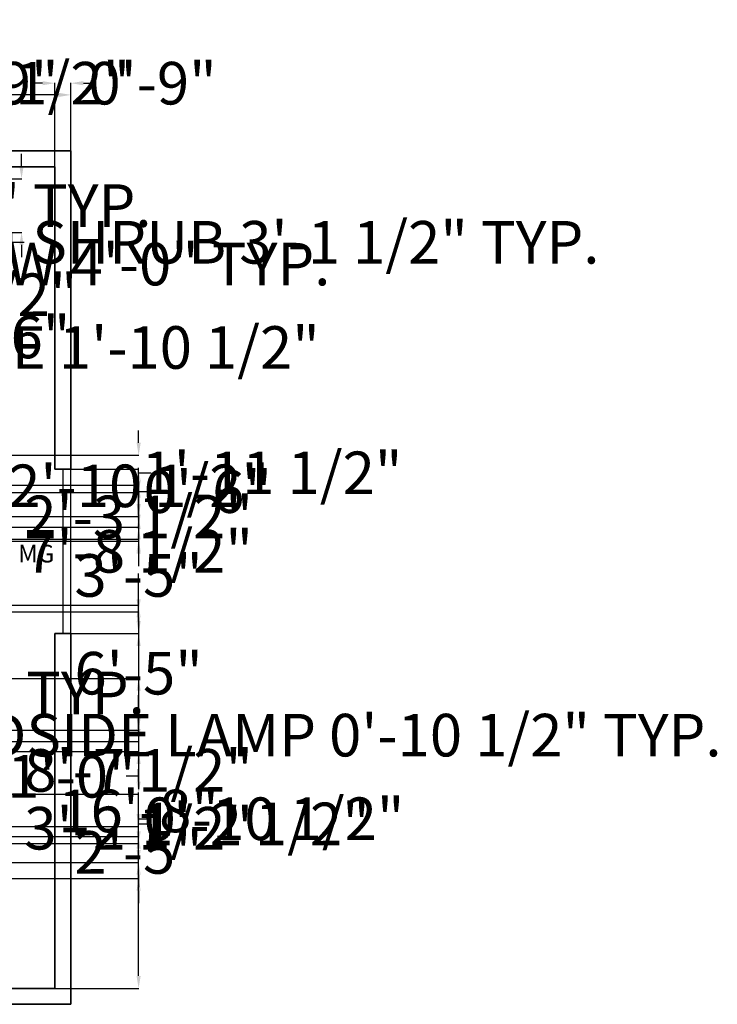
# Model space of a CAD drawing. Units: inches. Extents: x -166 to 1001, y 0 to 688.
# Tile 11 of 11: x 608 to 1001, y 74 to 629. Entities that reach past the tile are written whole.
import ezdxf

# ---------------------------------------------------------------- set-up
doc = ezdxf.new("R2010")
doc.units = ezdxf.units.IN
doc.header["$MEASUREMENT"] = 0
for name, color, linetype, lineweight in [('A-ANNO-DIMS', 1, 'Continuous', 18), ('A-ANNO-TEXT', 2, 'Continuous', 25), ('C-SITE-GATE', 250, 'Continuous', 25), ('C-SITE-WALL', 250, 'Continuous', 35)]:
    doc.layers.add(name, color=color, linetype=linetype, lineweight=lineweight)
doc.styles.get("Standard").update_dxf_attribs({"font": 'arial.ttf'})
doc.dimstyles.get("Standard").update_dxf_attribs({"dimtxt": 24, "dimasz": 7, "dimexe": 0.18, "dimexo": 0.0625, "dimgap": 0.09, "dimtad": 0, "dimtih": 1, "dimtoh": 1, "dimdec": 0, "dimzin": 0, "dimdsep": 46, "dimlunit": 3, "dimtxsty": 'Standard', "dimcen": 0.09, "dimadec": 0, "dimazin": 0, "dimtfac": 1, "dimtdec": 0, "dimtofl": 0, "dimtmove": 0, "dimatfit": 3, "dimfxl": 1, "dimtolj": 1, "dimtzin": 0, "dimarcsym": 0})

# ---------------------------------------------------------------- blocks, each defined once
blk = doc.blocks.new('*D10')
at = {"layer": 'A-ANNO-DIMS', "color": 0, "lineweight": -2, "transparency": 16777216}
for p, q in [((-82.62, 554.8), (-82.62, 586.48)), ((-75.62, 586.3), (256.61, 586.3)), ((629.88, 586.3), (297.65, 586.3)), ((636.88, 554.8), (636.88, 586.48))]:
    blk.add_line(p, q, dxfattribs=at)
at = {"layer": 'A-ANNO-DIMS', "color": 0, "transparency": 16777216}
for points in [[(-75.62, 587.47), (-75.62, 585.14), (-82.62, 586.3)], [(629.88, 587.47), (629.88, 585.14), (636.88, 586.3)]]:
    blk.add_solid(points, dxfattribs=at)
at = {"layer": 'Defpoints', "color": 0, "transparency": 16777216}
for p in [(636.88, 586.3), (-82.62, 554.74), (636.88, 554.74)]:
    blk.add_point(p, dxfattribs=at)
at = {"layer": 'A-ANNO-DIMS', "color": 0, "transparency": 16777216, "insert": (277.13, 586.3), "char_height": 24, "attachment_point": 5}
blk.add_mtext("\\A1;60'", dxfattribs=at)
blk = doc.blocks.new('*D15')
at = {"layer": 'A-ANNO-DIMS', "color": 0, "lineweight": -2, "transparency": 16777216}
for p, q in [((566.06, 508.76), (566.06, 503.04)), ((603.45, 508.76), (603.45, 503.04)), ((573.06, 503.22), (596.45, 503.22)), ((603.45, 503.22), (610.45, 503.22))]:
    blk.add_line(p, q, dxfattribs=at)
at = {"layer": 'A-ANNO-DIMS', "color": 0, "transparency": 16777216}
for points in [[(573.06, 504.38), (573.06, 502.05), (566.06, 503.22)], [(596.45, 504.38), (596.45, 502.05), (603.45, 503.22)]]:
    blk.add_solid(points, dxfattribs=at)
at = {"layer": 'Defpoints', "color": 0, "transparency": 16777216}
for p in [(566.06, 508.83), (603.45, 508.83), (603.45, 503.22)]:
    blk.add_point(p, dxfattribs=at)
at = {"layer": 'A-ANNO-DIMS', "color": 0, "transparency": 16777216, "insert": (774.93, 503.22), "char_height": 24, "attachment_point": 5}
blk.add_mtext('\\A1;SHRUB 3\'-1 1/2" TYP.', dxfattribs=at)
blk = doc.blocks.new('*D16')
at = {"layer": 'A-ANNO-DIMS', "color": 0, "lineweight": -2, "transparency": 16777216}
for p, q in [((609.06, 546), (609.06, 553)), ((603.51, 539), (609.24, 539)), ((603.51, 508.83), (609.24, 508.83)), ((609.06, 501.83), (609.06, 494.83))]:
    blk.add_line(p, q, dxfattribs=at)
at = {"layer": 'A-ANNO-DIMS', "color": 0, "transparency": 16777216}
for points in [[(607.89, 546), (610.23, 546), (609.06, 539)], [(607.89, 501.83), (610.23, 501.83), (609.06, 508.83)]]:
    blk.add_solid(points, dxfattribs=at)
at = {"layer": 'Defpoints', "color": 0, "transparency": 16777216}
for p in [(603.45, 539), (609.06, 539), (603.45, 508.83)]:
    blk.add_point(p, dxfattribs=at)
at = {"layer": 'A-ANNO-DIMS', "color": 0, "transparency": 16777216, "insert": (609.06, 523.91), "char_height": 24, "attachment_point": 5}
blk.add_mtext('\\A1;2\'-6" TYP.', dxfattribs=at)
blk = doc.blocks.new('*D17')
at = {"layer": 'A-ANNO-DIMS', "color": 0, "lineweight": -2, "transparency": 16777216}
for p, q in [((430.46, 483.8), (430.46, 491.12)), ((437.46, 490.94), (471.46, 490.94)), ((478.46, 483.8), (478.46, 491.12)), ((478.46, 490.94), (485.46, 490.94))]:
    blk.add_line(p, q, dxfattribs=at)
at = {"layer": 'A-ANNO-DIMS', "color": 0, "transparency": 16777216}
for points in [[(437.46, 492.11), (437.46, 489.77), (430.46, 490.94)], [(471.46, 492.11), (471.46, 489.77), (478.46, 490.94)]]:
    blk.add_solid(points, dxfattribs=at)
at = {"layer": 'Defpoints', "color": 0, "transparency": 16777216}
for p in [(478.46, 490.94), (430.46, 483.74), (478.46, 483.74)]:
    blk.add_point(p, dxfattribs=at)
at = {"layer": 'A-ANNO-DIMS', "color": 0, "transparency": 16777216, "insert": (637.4, 490.94), "char_height": 24, "attachment_point": 5}
blk.add_mtext('\\A1;WINDOW 4\'-0" TYP.', dxfattribs=at)
blk = doc.blocks.new('*D21')
at = {"layer": 'A-ANNO-DIMS', "color": 0, "lineweight": -2, "transparency": 16777216}
for p, q in [((506.04, 225.45), (499.04, 225.45)), ((513.04, 226.95), (513.04, 225.27)), ((523.44, 226.95), (523.44, 225.27)), ((530.44, 225.45), (537.44, 225.45))]:
    blk.add_line(p, q, dxfattribs=at)
at = {"layer": 'A-ANNO-DIMS', "color": 0, "transparency": 16777216}
for points in [[(506.04, 226.62), (506.04, 224.29), (513.04, 225.45)], [(530.44, 226.62), (530.44, 224.29), (523.44, 225.45)]]:
    blk.add_solid(points, dxfattribs=at)
at = {"layer": 'Defpoints', "color": 0, "transparency": 16777216}
for p in [(513.04, 227.01), (523.44, 227.01), (523.44, 225.45)]:
    blk.add_point(p, dxfattribs=at)
at = {"layer": 'A-ANNO-DIMS', "color": 0, "transparency": 16777216, "insert": (775.99, 225.45), "char_height": 24, "attachment_point": 5}
blk.add_mtext('\\A1;BEDSIDE LAMP 0\'-10 1/2" TYP.', dxfattribs=at)
blk = doc.blocks.new('*D22')
at = {"layer": 'A-ANNO-DIMS', "color": 0, "lineweight": -2, "transparency": 16777216}
for p, q in [((525, 242.21), (525, 249.21)), ((525, 249.21), (532, 249.21)), ((523.5, 235.21), (525.18, 235.21)), ((523.5, 227.01), (525.18, 227.01)), ((525, 220.01), (525, 213.01))]:
    blk.add_line(p, q, dxfattribs=at)
at = {"layer": 'A-ANNO-DIMS', "color": 0, "transparency": 16777216}
for points in [[(523.83, 242.21), (526.17, 242.21), (525, 235.21)], [(523.83, 220.01), (526.17, 220.01), (525, 227.01)]]:
    blk.add_solid(points, dxfattribs=at)
at = {"layer": 'Defpoints', "color": 0, "transparency": 16777216}
for p in [(523.44, 235.21), (525, 235.21), (523.44, 227.01)]:
    blk.add_point(p, dxfattribs=at)
at = {"layer": 'A-ANNO-DIMS', "color": 0, "transparency": 16777216, "insert": (605.24, 249.21), "char_height": 24, "attachment_point": 5}
blk.add_mtext('\\A1;0\'-8" TYP.', dxfattribs=at)
blk = doc.blocks.new('*D31')
at = {"layer": 'A-ANNO-DIMS', "color": 0, "lineweight": -2, "transparency": 16777216}
for p, q in [((484.56, 447.22), (484.56, 443.75)), ((506.92, 447.22), (506.92, 443.75)), ((491.56, 443.93), (499.92, 443.93)), ((506.92, 443.93), (513.92, 443.93))]:
    blk.add_line(p, q, dxfattribs=at)
at = {"layer": 'A-ANNO-DIMS', "color": 0, "transparency": 16777216}
for points in [[(491.56, 445.1), (491.56, 442.76), (484.56, 443.93)], [(499.92, 445.1), (499.92, 442.76), (506.92, 443.93)]]:
    blk.add_solid(points, dxfattribs=at)
at = {"layer": 'Defpoints', "color": 0, "transparency": 16777216}
for p in [(484.56, 447.28), (506.92, 447.28), (506.92, 443.93)]:
    blk.add_point(p, dxfattribs=at)
at = {"layer": 'A-ANNO-DIMS', "color": 0, "transparency": 16777216, "insert": (646.84, 443.93), "char_height": 24, "attachment_point": 5}
blk.add_mtext('\\A1;RANGE 1\'-10 1/2"', dxfattribs=at)
blk = doc.blocks.new('*D32')
at = {"layer": 'A-ANNO-DIMS', "color": 0, "lineweight": -2, "transparency": 16777216}
for p, q in [((510.27, 466.66), (510.27, 473.66)), ((510.27, 473.66), (517.27, 473.66)), ((506.98, 466.66), (510.45, 466.66)), ((510.27, 454.28), (510.27, 459.66)), ((506.98, 447.28), (510.45, 447.28))]:
    blk.add_line(p, q, dxfattribs=at)
at = {"layer": 'A-ANNO-DIMS', "color": 0, "transparency": 16777216}
for points in [[(509.1, 459.66), (511.44, 459.66), (510.27, 466.66)], [(509.1, 454.28), (511.44, 454.28), (510.27, 447.28)]]:
    blk.add_solid(points, dxfattribs=at)
at = {"layer": 'Defpoints', "color": 0, "transparency": 16777216}
for p in [(506.92, 466.66), (510.27, 466.66), (506.92, 447.28)]:
    blk.add_point(p, dxfattribs=at)
at = {"layer": 'A-ANNO-DIMS', "color": 0, "transparency": 16777216, "insert": (576.09, 473.66), "char_height": 24, "attachment_point": 5}
blk.add_mtext('\\A1;1\'-7 1/2"', dxfattribs=at)
blk = doc.blocks.new('*D33')
at = {"layer": 'A-ANNO-DIMS', "color": 0, "lineweight": -2, "transparency": 16777216}
for p, q in [((291.16, 438.23), (291.16, 450.03)), ((298.16, 449.85), (362.04, 449.85)), ((369.04, 438.23), (369.04, 450.03)), ((369.04, 449.85), (376.04, 449.85))]:
    blk.add_line(p, q, dxfattribs=at)
at = {"layer": 'A-ANNO-DIMS', "color": 0, "transparency": 16777216}
for points in [[(298.16, 451.02), (298.16, 448.68), (291.16, 449.85)], [(362.04, 451.02), (362.04, 448.68), (369.04, 449.85)]]:
    blk.add_solid(points, dxfattribs=at)
at = {"layer": 'Defpoints', "color": 0, "transparency": 16777216}
for p in [(369.04, 449.85), (291.16, 438.17), (369.04, 438.17)]:
    blk.add_point(p, dxfattribs=at)
at = {"layer": 'A-ANNO-DIMS', "color": 0, "transparency": 16777216, "insert": (508.03, 449.85), "char_height": 24, "attachment_point": 5}
blk.add_mtext('\\A1;DINING SET 6\'-6"', dxfattribs=at)
blk = doc.blocks.new('*D39')
at = {"layer": 'A-ANNO-DIMS', "color": 0, "lineweight": -2, "transparency": 16777216}
for p, q in [((627.94, 375.38), (675.21, 375.38)), ((675.03, 368.38), (675.03, 341.55)), ((675.03, 289.72), (675.03, 316.55)), ((627.94, 282.72), (675.21, 282.72))]:
    blk.add_line(p, q, dxfattribs=at)
at = {"layer": 'A-ANNO-DIMS', "color": 0, "transparency": 16777216}
for points in [[(673.87, 368.38), (676.2, 368.38), (675.03, 375.38)], [(673.87, 289.72), (676.2, 289.72), (675.03, 282.72)]]:
    blk.add_solid(points, dxfattribs=at)
at = {"layer": 'Defpoints', "color": 0, "transparency": 16777216}
for p in [(627.88, 375.38), (627.88, 282.72), (675.03, 282.72)]:
    blk.add_point(p, dxfattribs=at)
at = {"layer": 'A-ANNO-DIMS', "color": 0, "transparency": 16777216, "insert": (675.03, 329.05), "char_height": 24, "attachment_point": 5}
blk.add_mtext('\\A1;7\'-8 1/2"', dxfattribs=at)
blk = doc.blocks.new('*D40')
at = {"layer": 'A-ANNO-DIMS', "color": 0, "lineweight": -2, "transparency": 16777216}
for p, q in [((627.94, 282.72), (675.21, 282.72)), ((675.03, 275.72), (675.03, 195.07)), ((675.03, 89.74), (675.03, 170.38)), ((627.94, 82.74), (675.21, 82.74))]:
    blk.add_line(p, q, dxfattribs=at)
at = {"layer": 'A-ANNO-DIMS', "color": 0, "transparency": 16777216}
for points in [[(673.87, 275.72), (676.2, 275.72), (675.03, 282.72)], [(673.87, 89.74), (676.2, 89.74), (675.03, 82.74)]]:
    blk.add_solid(points, dxfattribs=at)
at = {"layer": 'Defpoints', "color": 0, "transparency": 16777216}
for p in [(627.88, 282.72), (675.03, 282.72), (627.88, 82.74)]:
    blk.add_point(p, dxfattribs=at)
at = {"layer": 'A-ANNO-DIMS', "color": 0, "transparency": 16777216, "insert": (675.03, 182.73), "char_height": 24, "attachment_point": 5}
blk.add_mtext('\\A1;16\'-8"', dxfattribs=at)
blk = doc.blocks.new('*D41')
at = {"layer": 'A-ANNO-DIMS', "color": 0, "lineweight": -2, "transparency": 16777216}
for p, q in [((620.88, 592.89), (613.88, 592.89)), ((627.88, 545.8), (627.88, 593.07)), ((636.88, 554.8), (636.88, 593.07)), ((643.88, 592.89), (650.88, 592.89))]:
    blk.add_line(p, q, dxfattribs=at)
at = {"layer": 'A-ANNO-DIMS', "color": 0, "transparency": 16777216}
for points in [[(620.88, 594.06), (620.88, 591.72), (627.88, 592.89)], [(643.88, 594.06), (643.88, 591.72), (636.88, 592.89)]]:
    blk.add_solid(points, dxfattribs=at)
at = {"layer": 'Defpoints', "color": 0, "transparency": 16777216}
for p in [(636.88, 592.89), (636.88, 554.74), (627.88, 545.74)]:
    blk.add_point(p, dxfattribs=at)
at = {"layer": 'A-ANNO-DIMS', "color": 0, "transparency": 16777216, "insert": (682.87, 592.89), "char_height": 24, "attachment_point": 5}
blk.add_mtext('\\A1;0\'-9"', dxfattribs=at)
blk = doc.blocks.new('*D47')
at = {"layer": 'A-ANNO-DIMS', "color": 0, "lineweight": -2, "transparency": 16777216}
for p, q in [((478.46, 483.8), (478.46, 593.07)), ((485.46, 592.89), (531.88, 592.89)), ((538.88, 483.8), (538.88, 593.07)), ((538.88, 592.89), (545.88, 592.89))]:
    blk.add_line(p, q, dxfattribs=at)
at = {"layer": 'A-ANNO-DIMS', "color": 0, "transparency": 16777216}
for points in [[(485.46, 594.06), (485.46, 591.72), (478.46, 592.89)], [(531.88, 594.06), (531.88, 591.72), (538.88, 592.89)]]:
    blk.add_solid(points, dxfattribs=at)
at = {"layer": 'Defpoints', "color": 0, "transparency": 16777216}
for p in [(538.88, 592.89), (478.46, 483.74), (538.88, 483.74)]:
    blk.add_point(p, dxfattribs=at)
at = {"layer": 'A-ANNO-DIMS', "color": 0, "transparency": 16777216, "insert": (605.83, 592.89), "char_height": 24, "attachment_point": 5}
blk.add_mtext('\\A1;5\'-0 1/2"', dxfattribs=at)
blk = doc.blocks.new('*D51')
at = {"layer": 'A-ANNO-DIMS', "color": 0, "lineweight": -2, "transparency": 16777216}
for p, q in [((675.03, 168.41), (675.03, 175.41)), ((675.03, 175.41), (682.03, 175.41)), ((24.44, 168.41), (675.21, 168.41)), ((675.03, 160.74), (675.03, 161.41)), ((24.44, 153.74), (675.21, 153.74))]:
    blk.add_line(p, q, dxfattribs=at)
at = {"layer": 'A-ANNO-DIMS', "color": 0, "transparency": 16777216}
for points in [[(673.87, 161.41), (676.2, 161.41), (675.03, 168.41)], [(673.87, 160.74), (676.2, 160.74), (675.03, 153.74)]]:
    blk.add_solid(points, dxfattribs=at)
at = {"layer": 'Defpoints', "color": 0, "transparency": 16777216}
for p in [(24.38, 168.41), (675.03, 168.41), (24.38, 153.74)]:
    blk.add_point(p, dxfattribs=at)
at = {"layer": 'A-ANNO-DIMS', "color": 0, "transparency": 16777216, "insert": (740.85, 175.41), "char_height": 24, "attachment_point": 5}
blk.add_mtext('\\A1;1\'-2 1/2"', dxfattribs=at)
blk = doc.blocks.new('*D52')
at = {"layer": 'A-ANNO-DIMS', "color": 0, "lineweight": -2, "transparency": 16777216}
for p, q in [((675.03, 366.29), (675.03, 373.29)), ((675.03, 373.29), (682.03, 373.29)), ((24.44, 366.29), (675.21, 366.29)), ((675.03, 349.74), (675.03, 359.29)), ((24.44, 342.74), (675.21, 342.74))]:
    blk.add_line(p, q, dxfattribs=at)
at = {"layer": 'A-ANNO-DIMS', "color": 0, "transparency": 16777216}
for points in [[(673.87, 359.29), (676.2, 359.29), (675.03, 366.29)], [(673.87, 349.74), (676.2, 349.74), (675.03, 342.74)]]:
    blk.add_solid(points, dxfattribs=at)
at = {"layer": 'Defpoints', "color": 0, "transparency": 16777216}
for p in [(24.38, 366.29), (675.03, 366.29), (24.38, 342.74)]:
    blk.add_point(p, dxfattribs=at)
at = {"layer": 'A-ANNO-DIMS', "color": 0, "transparency": 16777216, "insert": (750.18, 373.29), "char_height": 24, "attachment_point": 5}
blk.add_mtext('\\A1;1\'-11 1/2"', dxfattribs=at)
blk = doc.blocks.new('*D53')
at = {"layer": 'A-ANNO-DIMS', "color": 0, "lineweight": -2, "transparency": 16777216}
for p, q in [((675.03, 180.94), (675.03, 187.94)), ((538.94, 173.94), (675.21, 173.94)), ((538.94, 144.74), (675.21, 144.74)), ((675.03, 137.74), (675.03, 130.74))]:
    blk.add_line(p, q, dxfattribs=at)
at = {"layer": 'A-ANNO-DIMS', "color": 0, "transparency": 16777216}
for points in [[(673.87, 180.94), (676.2, 180.94), (675.03, 173.94)], [(673.87, 137.74), (676.2, 137.74), (675.03, 144.74)]]:
    blk.add_solid(points, dxfattribs=at)
at = {"layer": 'Defpoints', "color": 0, "transparency": 16777216}
for p in [(538.88, 173.94), (675.03, 173.94), (538.88, 144.74)]:
    blk.add_point(p, dxfattribs=at)
at = {"layer": 'A-ANNO-DIMS', "color": 0, "transparency": 16777216, "insert": (675.03, 159.34), "char_height": 24, "attachment_point": 5}
blk.add_mtext('\\A1;2\'-5"', dxfattribs=at)
blk = doc.blocks.new('*D54')
at = {"layer": 'A-ANNO-DIMS', "color": 0, "lineweight": -2, "transparency": 16777216}
for p, q in [((538.94, 298.79), (675.21, 298.79)), ((675.03, 291.79), (675.03, 272.71)), ((675.03, 228.94), (675.03, 248.02)), ((538.94, 221.94), (675.21, 221.94))]:
    blk.add_line(p, q, dxfattribs=at)
at = {"layer": 'A-ANNO-DIMS', "color": 0, "transparency": 16777216}
for points in [[(673.87, 291.79), (676.2, 291.79), (675.03, 298.79)], [(673.87, 228.94), (676.2, 228.94), (675.03, 221.94)]]:
    blk.add_solid(points, dxfattribs=at)
at = {"layer": 'Defpoints', "color": 0, "transparency": 16777216}
for p in [(538.88, 298.79), (675.03, 298.79), (538.88, 221.94)]:
    blk.add_point(p, dxfattribs=at)
at = {"layer": 'A-ANNO-DIMS', "color": 0, "transparency": 16777216, "insert": (675.03, 260.36), "char_height": 24, "attachment_point": 5}
blk.add_mtext('\\A1;6\'-5"', dxfattribs=at)
blk = doc.blocks.new('*D56')
at = {"layer": 'A-ANNO-DIMS', "color": 0, "lineweight": -2, "transparency": 16777216}
for p, q in [((675.03, 369.18), (675.03, 376.18)), ((538.94, 362.18), (675.21, 362.18)), ((538.94, 334.73), (675.21, 334.73)), ((675.03, 327.73), (675.03, 320.73))]:
    blk.add_line(p, q, dxfattribs=at)
at = {"layer": 'A-ANNO-DIMS', "color": 0, "transparency": 16777216}
for points in [[(673.87, 369.18), (676.2, 369.18), (675.03, 362.18)], [(673.87, 327.73), (676.2, 327.73), (675.03, 334.73)]]:
    blk.add_solid(points, dxfattribs=at)
at = {"layer": 'Defpoints', "color": 0, "transparency": 16777216}
for p in [(538.88, 362.18), (675.03, 362.18), (538.88, 334.73)]:
    blk.add_point(p, dxfattribs=at)
at = {"layer": 'A-ANNO-DIMS', "color": 0, "transparency": 16777216, "insert": (675.03, 348.46), "char_height": 24, "attachment_point": 5}
blk.add_mtext('\\A1;2\'-3 1/2"', dxfattribs=at)
blk = doc.blocks.new('*D57')
at = {"layer": 'A-ANNO-DIMS', "color": 0, "lineweight": -2, "transparency": 16777216}
for p, q in [((531.88, 592.89), (524.88, 592.89)), ((538.88, 335.97), (538.88, 593.07)), ((547.76, 325.77), (547.76, 593.07)), ((554.76, 592.89), (561.76, 592.89))]:
    blk.add_line(p, q, dxfattribs=at)
at = {"layer": 'A-ANNO-DIMS', "color": 0, "transparency": 16777216}
for points in [[(531.88, 594.06), (531.88, 591.72), (538.88, 592.89)], [(554.76, 594.06), (554.76, 591.72), (547.76, 592.89)]]:
    blk.add_solid(points, dxfattribs=at)
at = {"layer": 'Defpoints', "color": 0, "transparency": 16777216}
for p in [(547.76, 592.89), (538.88, 335.91), (547.76, 325.71)]:
    blk.add_point(p, dxfattribs=at)
at = {"layer": 'A-ANNO-DIMS', "color": 0, "transparency": 16777216, "insert": (593.75, 592.89), "char_height": 24, "attachment_point": 5}
blk.add_mtext('\\A1;0\'-9"', dxfattribs=at)
blk = doc.blocks.new('*D58')
at = {"layer": 'A-ANNO-DIMS', "color": 0, "lineweight": -2, "transparency": 16777216}
for p, q in [((542.41, 335.91), (675.21, 335.91)), ((675.03, 328.91), (675.03, 327.8)), ((675.03, 301.99), (675.03, 303.1)), ((542.41, 294.99), (675.21, 294.99))]:
    blk.add_line(p, q, dxfattribs=at)
at = {"layer": 'A-ANNO-DIMS', "color": 0, "transparency": 16777216}
for points in [[(673.87, 328.91), (676.2, 328.91), (675.03, 335.91)], [(673.87, 301.99), (676.2, 301.99), (675.03, 294.99)]]:
    blk.add_solid(points, dxfattribs=at)
at = {"layer": 'Defpoints', "color": 0, "transparency": 16777216}
for p in [(542.35, 335.91), (542.35, 294.99), (675.03, 294.99)]:
    blk.add_point(p, dxfattribs=at)
at = {"layer": 'A-ANNO-DIMS', "color": 0, "transparency": 16777216, "insert": (675.03, 315.45), "char_height": 24, "attachment_point": 5}
blk.add_mtext('\\A1;3\'-5"', dxfattribs=at)
blk = doc.blocks.new('*D65')
at = {"layer": 'A-ANNO-DIMS', "color": 0, "lineweight": -2, "transparency": 16777216}
for p, q in [((675.03, 390.21), (675.03, 397.21)), ((397.94, 383.21), (675.21, 383.21)), ((397.94, 348.69), (675.21, 348.69)), ((675.03, 341.69), (675.03, 334.69))]:
    blk.add_line(p, q, dxfattribs=at)
at = {"layer": 'A-ANNO-DIMS', "color": 0, "transparency": 16777216}
for points in [[(673.87, 390.21), (676.2, 390.21), (675.03, 383.21)], [(673.87, 341.69), (676.2, 341.69), (675.03, 348.69)]]:
    blk.add_solid(points, dxfattribs=at)
at = {"layer": 'Defpoints', "color": 0, "transparency": 16777216}
for p in [(397.88, 383.21), (675.03, 383.21), (397.88, 348.69)]:
    blk.add_point(p, dxfattribs=at)
at = {"layer": 'A-ANNO-DIMS', "color": 0, "transparency": 16777216, "insert": (675.03, 365.95), "char_height": 24, "attachment_point": 5}
blk.add_mtext('\\A1;2\'-10 1/2"', dxfattribs=at)
blk = doc.blocks.new('*D66')
at = {"layer": 'A-ANNO-DIMS', "color": 0, "lineweight": -2, "transparency": 16777216}
for p, q in [((675.03, 355.69), (675.03, 362.69)), ((675.03, 362.69), (682.03, 362.69)), ((397.94, 348.69), (675.21, 348.69)), ((397.94, 342.74), (675.21, 342.74)), ((675.03, 335.74), (675.03, 328.74))]:
    blk.add_line(p, q, dxfattribs=at)
at = {"layer": 'A-ANNO-DIMS', "color": 0, "transparency": 16777216}
for points in [[(673.87, 355.69), (676.2, 355.69), (675.03, 348.69)], [(673.87, 335.74), (676.2, 335.74), (675.03, 342.74)]]:
    blk.add_solid(points, dxfattribs=at)
at = {"layer": 'Defpoints', "color": 0, "transparency": 16777216}
for p in [(397.88, 348.69), (675.03, 348.69), (397.88, 342.74)]:
    blk.add_point(p, dxfattribs=at)
at = {"layer": 'A-ANNO-DIMS', "color": 0, "transparency": 16777216, "insert": (714.02, 362.69), "char_height": 24, "attachment_point": 5}
blk.add_mtext('\\A1;0\'-6"', dxfattribs=at)
blk = doc.blocks.new('*D74')
at = {"layer": 'A-ANNO-DIMS', "color": 0, "lineweight": -2, "transparency": 16777216}
for p, q in [((675.03, 171.32), (675.03, 178.32)), ((675.03, 178.32), (682.03, 178.32)), ((397.94, 164.32), (675.21, 164.32)), ((397.94, 153.74), (675.21, 153.74)), ((675.03, 146.74), (675.03, 139.74))]:
    blk.add_line(p, q, dxfattribs=at)
at = {"layer": 'A-ANNO-DIMS', "color": 0, "transparency": 16777216}
for points in [[(673.87, 171.32), (676.2, 171.32), (675.03, 164.32)], [(673.87, 146.74), (676.2, 146.74), (675.03, 153.74)]]:
    blk.add_solid(points, dxfattribs=at)
at = {"layer": 'Defpoints', "color": 0, "transparency": 16777216}
for p in [(397.88, 164.32), (675.03, 164.32), (397.88, 153.74)]:
    blk.add_point(p, dxfattribs=at)
at = {"layer": 'A-ANNO-DIMS', "color": 0, "transparency": 16777216, "insert": (751.31, 178.32), "char_height": 24, "attachment_point": 5}
blk.add_mtext('\\A1;0\'-10 1/2"', dxfattribs=at)
blk = doc.blocks.new('*D76')
at = {"layer": 'A-ANNO-DIMS', "color": 0, "lineweight": -2, "transparency": 16777216}
for p, q in [((675.03, 235.24), (675.03, 242.24)), ((160.94, 228.24), (675.21, 228.24)), ((160.94, 216.24), (675.21, 216.24)), ((675.03, 209.24), (675.03, 202.24)), ((675.03, 202.24), (668.03, 202.24))]:
    blk.add_line(p, q, dxfattribs=at)
at = {"layer": 'A-ANNO-DIMS', "color": 0, "transparency": 16777216}
for points in [[(673.87, 235.24), (676.2, 235.24), (675.03, 228.24)], [(673.87, 209.24), (676.2, 209.24), (675.03, 216.24)]]:
    blk.add_solid(points, dxfattribs=at)
at = {"layer": 'Defpoints', "color": 0, "transparency": 16777216}
for p in [(160.88, 228.24), (160.88, 216.24), (675.03, 216.24)]:
    blk.add_point(p, dxfattribs=at)
at = {"layer": 'A-ANNO-DIMS', "color": 0, "transparency": 16777216, "insert": (637.17, 202.24), "char_height": 24, "attachment_point": 5}
blk.add_mtext('\\A1;1\'-0"', dxfattribs=at)
blk = doc.blocks.new('*D77')
at = {"layer": 'A-ANNO-DIMS', "color": 0, "lineweight": -2, "transparency": 16777216}
for p, q in [((675.03, 199.24), (675.03, 206.24)), ((292.83, 192.24), (675.21, 192.24)), ((292.83, 153.74), (675.21, 153.74)), ((675.03, 146.74), (675.03, 139.74))]:
    blk.add_line(p, q, dxfattribs=at)
at = {"layer": 'A-ANNO-DIMS', "color": 0, "transparency": 16777216}
for points in [[(673.87, 199.24), (676.2, 199.24), (675.03, 192.24)], [(673.87, 146.74), (676.2, 146.74), (675.03, 153.74)]]:
    blk.add_solid(points, dxfattribs=at)
at = {"layer": 'Defpoints', "color": 0, "transparency": 16777216}
for p in [(292.77, 192.24), (292.77, 153.74), (675.03, 153.74)]:
    blk.add_point(p, dxfattribs=at)
at = {"layer": 'A-ANNO-DIMS', "color": 0, "transparency": 16777216, "insert": (675.03, 172.99), "char_height": 24, "attachment_point": 5}
blk.add_mtext('\\A1;3\'-2 1/2"', dxfattribs=at)
blk = doc.blocks.new('*D79')
at = {"layer": 'A-ANNO-DIMS', "color": 0, "lineweight": -2, "transparency": 16777216}
for p, q in [((208.68, 257.42), (675.21, 257.42)), ((675.03, 250.42), (675.03, 218.08)), ((675.03, 160.74), (675.03, 193.08)), ((292.83, 153.74), (675.21, 153.74))]:
    blk.add_line(p, q, dxfattribs=at)
at = {"layer": 'A-ANNO-DIMS', "color": 0, "transparency": 16777216}
for points in [[(673.87, 250.42), (676.2, 250.42), (675.03, 257.42)], [(673.87, 160.74), (676.2, 160.74), (675.03, 153.74)]]:
    blk.add_solid(points, dxfattribs=at)
at = {"layer": 'Defpoints', "color": 0, "transparency": 16777216}
for p in [(208.62, 257.42), (292.77, 153.74), (675.03, 153.74)]:
    blk.add_point(p, dxfattribs=at)
at = {"layer": 'A-ANNO-DIMS', "color": 0, "transparency": 16777216, "insert": (675.03, 205.58), "char_height": 24, "attachment_point": 5}
blk.add_mtext('\\A1;8\'-7 1/2"', dxfattribs=at)

msp = doc.modelspace()

# ---------------------------------------------------------------- linework, layer by layer
at = {"layer": 'C-SITE-GATE'}
msp.add_lwpolyline([(636.88, 375.38), (632.38, 375.38), (632.38, 282.72), (636.88, 282.72)], close=True, dxfattribs=at)
at = {"layer": 'C-SITE-WALL'}
for p, q in [((-82.62, 554.74), (636.88, 554.74)), ((636.88, 375.38), (636.88, 554.74)), ((-73.62, 545.74), (627.88, 545.74)), ((627.88, 375.38), (627.88, 545.74)), ((627.88, 375.38), (636.88, 375.38)), ((627.88, 82.74), (627.88, 282.72)), ((627.88, 282.72), (636.88, 282.72)), ((636.88, 73.74), (636.88, 282.72)), ((-73.62, 82.74), (627.88, 82.74)), ((-82.62, 73.74), (636.88, 73.74))]:
    msp.add_line(p, q, dxfattribs=at)

# ---------------------------------------------------------------- texts
at = {"layer": 'A-ANNO-TEXT'}
msp.add_text('MG', height=9.972, dxfattribs=at).set_placement((607.11, 322.75))

# ---------------------------------------------------------------- dimensions: what is measured, and where the dimension line sits
at = {"layer": 'A-ANNO-DIMS'}
for base, p1, p2, override, picture, middle in [((538.88, 592.89), (478.46, 483.74), (538.88, 483.74), {"dimdec": 1, "dimlfac": 1, "dimrnd": 0, "dimzin": 1, "dimdsep": 46, "dimlunit": 4, "dimfrac": 2}, '*D47', (605.83, 592.89)), ((547.76, 592.89), (538.88, 335.91), (547.76, 325.71), {"dimdec": 1, "dimlfac": 1, "dimrnd": 0, "dimzin": 1, "dimdsep": 46, "dimlunit": 4, "dimfrac": 2}, '*D57', (593.75, 592.89)), ((636.88, 592.89), (627.88, 545.74), (636.88, 554.74), {"dimdec": 1, "dimlfac": 1, "dimrnd": 0, "dimzin": 1, "dimdsep": 46, "dimlunit": 4, "dimfrac": 2}, '*D41', (682.87, 592.89)), ((636.88246038, 586.30455527), (-82.61753962, 554.740867), (636.88246038, 554.740867), {"dimclrd": 0, "dimclre": 0, "dimclrt": 0}, '*D10', (277.13246038, 586.30455527))]:
    dim = msp.add_linear_dim(base=base, p1=p1, p2=p2, dimstyle='Standard', override=override, dxfattribs=at)
    dim.commit()
    dim.dimension.update_dxf_attribs({"geometry": picture, "text_midpoint": middle})
for base, p1, p2, text, picture, middle in [((603.45, 503.22), (566.06, 508.83), (603.45, 508.83), 'SHRUB <> TYP.', '*D15', (774.93, 503.22)), ((478.46, 490.94), (430.46, 483.74), (478.46, 483.74), 'WINDOW <> TYP.', '*D17', (637.4, 490.94)), ((369.04, 449.85), (291.16, 438.17), (369.04, 438.17), 'DINING SET <>', '*D33', (508.03, 449.85)), ((506.92, 443.93), (484.56, 447.28), (506.92, 447.28), 'RANGE <>', '*D31', (646.84, 443.93)), ((523.44, 225.45), (513.04, 227.01), (523.44, 227.01), 'BEDSIDE LAMP <> TYP.', '*D21', (775.99, 225.45))]:
    dim = msp.add_linear_dim(base=base, p1=p1, p2=p2, text=text, dimstyle='Standard', override={"dimdec": 1, "dimlfac": 1, "dimrnd": 0, "dimzin": 1, "dimdsep": 46, "dimlunit": 4, "dimfrac": 2}, dxfattribs=at)
    dim.commit()
    dim.dimension.update_dxf_attribs({"geometry": picture, "text_midpoint": middle})
for base, p1, p2, picture, middle in [((609.06, 539), (603.45, 508.83), (603.45, 539), '*D16', (609.06, 523.91)), ((525, 235.21), (523.44, 227.01), (523.44, 235.21), '*D22', (605.24, 249.21))]:
    dim = msp.add_linear_dim(base=base, p1=p1, p2=p2, angle=90, text='<> TYP.', dimstyle='Standard', override={"dimdec": 1, "dimlfac": 1, "dimrnd": 0, "dimzin": 1, "dimdsep": 46, "dimlunit": 4, "dimfrac": 2}, dxfattribs=at)
    dim.commit()
    dim.dimension.update_dxf_attribs({"geometry": picture, "text_midpoint": middle})
for base, p1, p2, picture, middle in [((510.27, 466.66), (506.92, 447.28), (506.92, 466.66), '*D32', (576.09, 473.66)), ((675.0325, 366.2884), (24.3825, 342.7409), (24.3825, 366.2884), '*D52', (750.177, 373.2884)), ((675.03, 383.21), (397.88, 348.69), (397.88, 383.21), '*D65', (675.03, 365.95)), ((675.0325, 362.1777), (538.8825, 334.734), (538.8825, 362.1777), '*D56', (675.0325, 348.4559)), ((675.0325, 348.6892), (397.8825, 342.7409), (397.8825, 348.6892), '*D66', (714.0215, 362.6892)), ((675.03, 282.72), (627.88, 375.38), (627.88, 282.72), '*D39', (675.03, 329.05)), ((675.03, 294.99), (542.35, 335.91), (542.35, 294.99), '*D58', (675.03, 315.45)), ((675.0325, 298.7872), (538.8825, 221.9421), (538.8825, 298.7872), '*D54', (675.0325, 260.3646)), ((675.03, 282.72), (627.88, 82.74), (627.88, 282.72), '*D40', (675.03, 182.73)), ((675.03, 153.74), (208.62, 257.42), (292.77, 153.74), '*D79', (675.03, 205.58)), ((675.03, 216.24), (160.88, 228.24), (160.88, 216.24), '*D76', (637.17, 202.24)), ((675.03, 168.41), (24.38, 153.74), (24.38, 168.41), '*D51', (740.85, 175.41)), ((675.03, 164.32), (397.88, 153.74), (397.88, 164.32), '*D74', (751.31, 178.32)), ((675.03, 153.74), (292.77, 192.24), (292.77, 153.74), '*D77', (675.03, 172.99)), ((675.03, 173.94), (538.88, 144.74), (538.88, 173.94), '*D53', (675.03, 159.34))]:
    dim = msp.add_linear_dim(base=base, p1=p1, p2=p2, angle=90, dimstyle='Standard', override={"dimdec": 1, "dimlfac": 1, "dimrnd": 0, "dimzin": 1, "dimdsep": 46, "dimlunit": 4, "dimfrac": 2}, dxfattribs=at)
    dim.commit()
    dim.dimension.update_dxf_attribs({"geometry": picture, "text_midpoint": middle})

doc.saveas('drawing.dxf')
